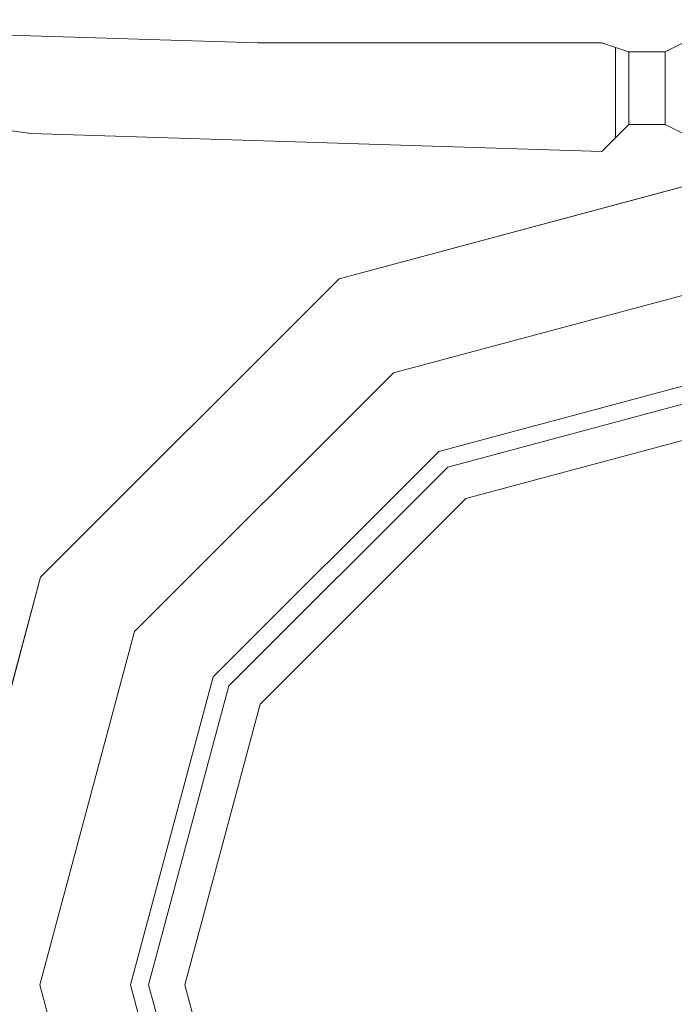
# Model space of a CAD drawing. Units: inches. Extents: x 375 to 1122, y 27 to 1069.
# Tile 35 of 155: x 734.833 to 739.279, y 277.109 to 283.8. Entities that reach past the tile are written whole.
import ezdxf

# ---------------------------------------------------------------- set-up
doc = ezdxf.new("R2010")
doc.units = ezdxf.units.IN
doc.layers.add('A-ANNO-DIMS', color=2, linetype='Continuous', lineweight=18)
doc.layers.add('Furniture', color=30, linetype='Continuous', lineweight=18)
doc.styles.get("Standard").update_dxf_attribs({"font": 'arial.ttf'})
doc.dimstyles.new('ISO-25', dxfattribs={"dimtxt": 12, "dimasz": 2.5, "dimexe": 1.5, "dimexo": 1.5, "dimtad": 1, "dimdec": 1, "dimlunit": 3, "dimtxsty": 'Standard', "dimblk": 'ARCHTICK', "dimcen": 2.5, "dimadec": 0, "dimazin": 0, "dimtfac": 1, "dimtdec": 1, "dimtmove": 0, "dimatfit": 3, "dimfxl": 1.5, "dimfxlon": 1, "dimarcsym": 0})

# ---------------------------------------------------------------- blocks, each defined once
blk = doc.blocks.new('A$C403C54AD')
at = {"linetype": 'ByBlock', "invisible_edges": 5}
for points in [[(1.58798, 1.37069, -0.02349), (1.60645, 1.37069, -0.02349), (1.62254, 1.31066, -0.02349), (1.60654, 1.30143, -0.02349)], [(1.62185, 1.37069, -0.03734), (1.58798, 1.37069, -0.02811), (1.60654, 1.30143, -0.02811), (1.63587, 1.31836, -0.03734)], [(1.60645, 1.37069, -0.02349), (1.62492, 1.37069, -0.02965), (1.63853, 1.3199, -0.02965), (1.62254, 1.31066, -0.02349)], [(1.63108, 1.37069, -0.04658), (1.62185, 1.37069, -0.03734), (1.63587, 1.31836, -0.03734), (1.64387, 1.32297, -0.04658)], [(1.62492, 1.37069, -0.02965), (1.72651, 1.37069, -0.02965), (1.72651, 1.37069, -0.02965), (1.63853, 1.3199, -0.02965)], [(1.63853, 1.3199, -0.02965), (1.72651, 1.37069, -0.02965), (1.72651, 1.37069, -0.02965), (1.67572, 1.28271, -0.02965)], [(1.67572, 1.28271, -0.02965), (1.72651, 1.37069, -0.02965), (1.72651, 1.37069, -0.02965), (1.72651, 1.2691, -0.02965)], [(1.72651, 1.2691, -0.02965), (1.72651, 1.37069, -0.02965), (1.72651, 1.37069, -0.02965), (1.7773, 1.28271, -0.02965)], [(1.81449, 1.3199, -0.02965), (1.72651, 1.37069, -0.02965), (1.72651, 1.37069, -0.02965), (1.8281, 1.37069, -0.02965)], [(1.7773, 1.28271, -0.02965), (1.72651, 1.37069, -0.02965), (1.72651, 1.37069, -0.02965), (1.81449, 1.3199, -0.02965)], [(1.64387, 1.32297, -0.04658), (1.63587, 1.31836, -0.03734), (1.67418, 1.28005, -0.03734), (1.6788, 1.28804, -0.04658)], [(1.62254, 1.31066, -0.02349), (1.63853, 1.3199, -0.02965), (1.67572, 1.28271, -0.02965), (1.66648, 1.26672, -0.02349)], [(1.63587, 1.31836, -0.03734), (1.60654, 1.30143, -0.02811), (1.65725, 1.25072, -0.02811), (1.67418, 1.28005, -0.03734)], [(1.60654, 1.30143, -0.02349), (1.62254, 1.31066, -0.02349), (1.66648, 1.26672, -0.02349), (1.65725, 1.25072, -0.02349)], [(1.6788, 1.28804, -0.04658), (1.67418, 1.28005, -0.03734), (1.72651, 1.26602, -0.03734), (1.72651, 1.27526, -0.04658)], [(1.72651, 1.27526, -0.04658), (1.72651, 1.26602, -0.03734), (1.77884, 1.28005, -0.03734), (1.77423, 1.28804, -0.04658)], [(1.66648, 1.26672, -0.02349), (1.67572, 1.28271, -0.02965), (1.72651, 1.2691, -0.02965), (1.72651, 1.25063, -0.02349)], [(1.72651, 1.25063, -0.02349), (1.72651, 1.2691, -0.02965), (1.7773, 1.28271, -0.02965), (1.78654, 1.26672, -0.02349)], [(1.67418, 1.28005, -0.03734), (1.65725, 1.25072, -0.02811), (1.72651, 1.23216, -0.02811), (1.72651, 1.26602, -0.03734)], [(1.72651, 1.26602, -0.03734), (1.72651, 1.23216, -0.02811), (1.79578, 1.25072, -0.02811), (1.77884, 1.28005, -0.03734)], [(1.65725, 1.25072, -0.02349), (1.66648, 1.26672, -0.02349), (1.72651, 1.25063, -0.02349), (1.72651, 1.23216, -0.02349)], [(1.72651, 1.23216, -0.02349), (1.72651, 1.25063, -0.02349), (1.78654, 1.26672, -0.02349), (1.79578, 1.25072, -0.02349)]]:
    blk.add_3dface(points, dxfattribs=at)
at = {"linetype": 'ByBlock'}
for points in [[(1.58798, 1.37069, -0.02811), (1.58798, 1.37069, -0.02349), (1.60654, 1.30143, -0.02349), (1.60654, 1.30143, -0.02811)], [(1.60654, 1.30143, -0.02811), (1.60654, 1.30143, -0.02349), (1.65725, 1.25072, -0.02349), (1.65725, 1.25072, -0.02811)], [(1.65725, 1.25072, -0.02811), (1.65725, 1.25072, -0.02349), (1.72651, 1.23216, -0.02349), (1.72651, 1.23216, -0.02811)], [(1.72651, 1.23216, -0.02811), (1.72651, 1.23216, -0.02349), (1.79578, 1.25072, -0.02349), (1.79578, 1.25072, -0.02811)]]:
    blk.add_3dface(points, dxfattribs=at)
for points in [[(1.58029, 1.35684, -0.03581), (1.56797, 1.35684, -0.03581), (1.56644, 1.35991, -0.03427), (1.58183, 1.35991, -0.03427)], [(1.58029, 1.35684, -0.04504), (1.56797, 1.35684, -0.04504), (1.56644, 1.35991, -0.04658), (1.58183, 1.35991, -0.04658)], [(1.56644, 1.35991, -0.03427), (1.56644, 1.35991, -0.04658), (1.56797, 1.35684, -0.04504), (1.56797, 1.35684, -0.03581)], [(1.58029, 1.35684, -0.03581), (1.58029, 1.35684, -0.04504), (1.58183, 1.35991, -0.04658), (1.58183, 1.35991, -0.03427)], [(1.56797, 1.35068, -0.03581), (1.58029, 1.35068, -0.03581), (1.58029, 1.35684, -0.03581), (1.56797, 1.35684, -0.03581)], [(1.56797, 1.35068, -0.04504), (1.58029, 1.35068, -0.04504), (1.58029, 1.35684, -0.04504), (1.56797, 1.35684, -0.04504)], [(1.5826, 1.34837, -0.03888), (1.56721, 1.34837, -0.03888), (1.56797, 1.35068, -0.03581), (1.58029, 1.35068, -0.03581)], [(1.5826, 1.34837, -0.04196), (1.56721, 1.34837, -0.04196), (1.56797, 1.35068, -0.04504), (1.58029, 1.35068, -0.04504)]]:
    blk.add_3dface(points)
for points, invisible_edges in [([(1.56797, 1.35684, -0.04504), (1.56797, 1.35684, -0.03581), (1.56797, 1.35068, -0.03581), (1.56797, 1.35068, -0.04504)], 4), ([(1.58029, 1.35068, -0.04504), (1.58029, 1.35068, -0.03581), (1.58029, 1.35684, -0.03581), (1.58029, 1.35684, -0.04504)], 1), ([(1.56797, 1.35068, -0.03581), (1.56797, 1.35068, -0.04504), (1.56721, 1.34837, -0.04196), (1.56721, 1.34837, -0.03888)], 5), ([(1.5826, 1.34837, -0.03888), (1.5826, 1.34837, -0.04196), (1.58029, 1.35068, -0.04504), (1.58029, 1.35068, -0.03581)], 5), ([(1.58491, 1.34606, -0.03965), (1.56644, 1.34606, -0.03965), (1.56721, 1.34837, -0.03888), (1.5826, 1.34837, -0.03888)], 1), ([(1.58491, 1.34606, -0.04119), (1.56644, 1.34606, -0.04119), (1.56721, 1.34837, -0.04196), (1.5826, 1.34837, -0.04196)], 1), ([(1.56721, 1.34837, -0.04196), (1.56721, 1.34837, -0.03888), (1.56644, 1.34606, -0.03965), (1.56644, 1.34606, -0.04119)], 5), ([(1.58491, 1.34606, -0.04119), (1.58491, 1.34606, -0.03965), (1.5826, 1.34837, -0.03888), (1.5826, 1.34837, -0.04196)], 5), ([(1.56644, 1.28757, -0.03965), (1.58183, 1.24909, -0.03965), (1.58491, 1.34606, -0.03965), (1.56644, 1.34606, -0.03965)], 5), ([(1.56644, 1.28757, -0.04119), (1.58183, 1.24909, -0.04119), (1.58491, 1.34606, -0.04119), (1.56644, 1.34606, -0.04119)], 5), ([(1.56644, 1.34606, -0.03965), (1.56644, 1.34606, -0.04119), (1.56644, 1.28757, -0.04119), (1.56644, 1.28757, -0.03965)], 5), ([(1.58183, 1.24909, -0.04119), (1.58183, 1.24909, -0.03965), (1.58491, 1.34606, -0.03965), (1.58491, 1.34606, -0.04119)], 5), ([(1.58029, 1.23832, -0.03965), (1.5649, 1.23832, -0.03965), (1.56644, 1.28757, -0.03965), (1.58183, 1.24909, -0.03965)], 5), ([(1.58029, 1.23832, -0.04119), (1.5649, 1.23832, -0.04119), (1.56644, 1.28757, -0.04119), (1.58183, 1.24909, -0.04119)], 5), ([(1.56644, 1.28757, -0.04119), (1.56644, 1.28757, -0.03965), (1.5649, 1.23832, -0.03965), (1.5649, 1.23832, -0.04119)], 5), ([(1.58029, 1.23832, -0.03965), (1.58029, 1.23832, -0.04119), (1.58183, 1.24909, -0.04119), (1.58183, 1.24909, -0.03965)], 5)]:
    blk.add_3dface(points, dxfattribs=dict(invisible_edges=invisible_edges))
blk = doc.blocks.new('_ArchTick')
at = {"color": 0, "linetype": 'ByBlock', "const_width": 0.15}
blk.add_lwpolyline([(-0.5, -0.5), (0.5, 0.5)], dxfattribs=at)
blk = doc.blocks.new('*D94')
at = {"layer": 'A-ANNO-DIMS', "color": 0, "lineweight": -2, "transparency": 16777216}
for p, q in [((734.0073, 117.5277), (734.0073, 114.5277)), ((773.0073, 117.5277), (773.0073, 114.5277)), ((734.0073, 116.0277), (773.0073, 116.0277))]:
    blk.add_line(p, q, dxfattribs=at)
at = {"layer": 'Defpoints', "color": 0, "transparency": 16777216}
for p in [(734.0073, 667.5277), (773.0073, 667.5277), (773.0073, 116.0277)]:
    blk.add_point(p, dxfattribs=at)
at = {"layer": 'A-ANNO-DIMS', "color": 0, "lineweight": -2, "transparency": 16777216, "xscale": 2.5, "yscale": 2.5, "zscale": 2.5, "rotation": 180}
blk.add_blockref('_ArchTick', (734.0073, 116.0277), dxfattribs=at)
at = {"layer": 'A-ANNO-DIMS', "color": 0, "lineweight": -2, "transparency": 16777216, "xscale": 2.5, "yscale": 2.5, "zscale": 2.5}
blk.add_blockref('_ArchTick', (773.0073, 116.0277), dxfattribs=at)
at = {"layer": 'A-ANNO-DIMS', "color": 0, "transparency": 16777216, "insert": (753.5073, 122.7837), "char_height": 12, "attachment_point": 5}
blk.add_mtext('3\'-3"', dxfattribs=at)

msp = doc.modelspace()

# ---------------------------------------------------------------- block references
at = {"layer": 'Furniture', "xscale": 39.9918517141215, "yscale": 39.9918517141215, "zscale": 39.9918517141215, "rotation": 270}
msp.add_blockref('A$C403C54AD', (684.9549, 346.2875, 0.024), dxfattribs=at)

# ---------------------------------------------------------------- dimensions: what is measured, and where the dimension line sits
at = {"layer": 'A-ANNO-DIMS'}
dim = msp.add_linear_dim(base=(773.0073, 116.0277), p1=(734.0073, 667.5277), p2=(773.0073, 667.5277), dimstyle='ISO-25', override={"dimdec": 1, "dimlfac": 1, "dimrnd": 0, "dimzin": 1, "dimdsep": 46, "dimlunit": 4, "dimfrac": 2}, dxfattribs=at)
dim.commit()
dim.dimension.update_dxf_attribs({"geometry": '*D94', "text_midpoint": (753.5073, 122.7837)})

doc.saveas('drawing.dxf')
